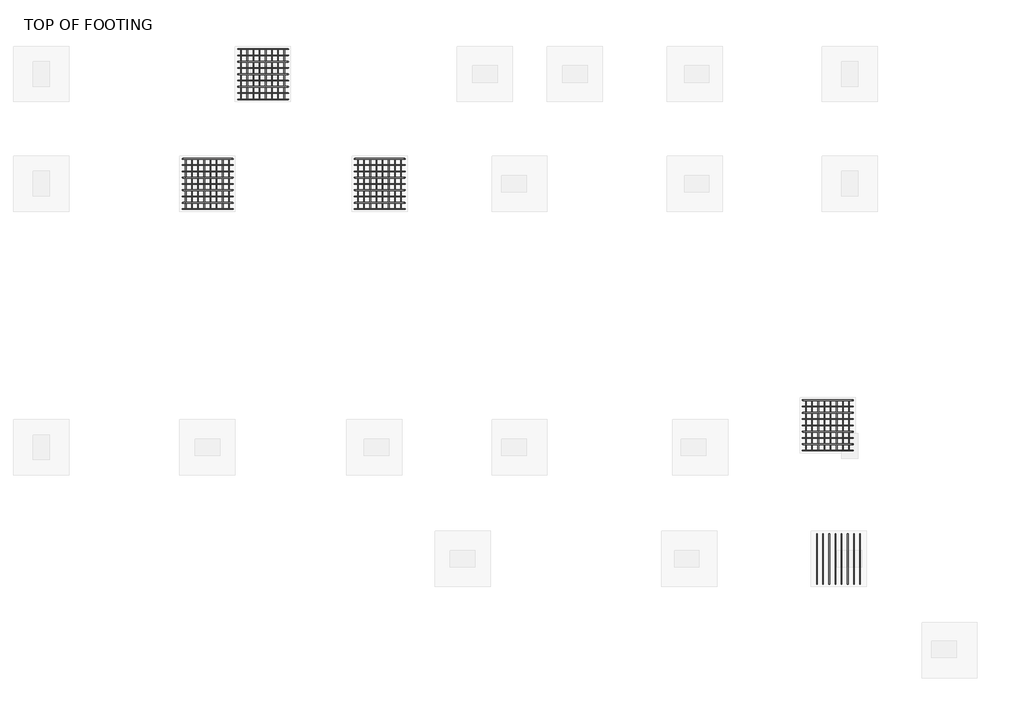
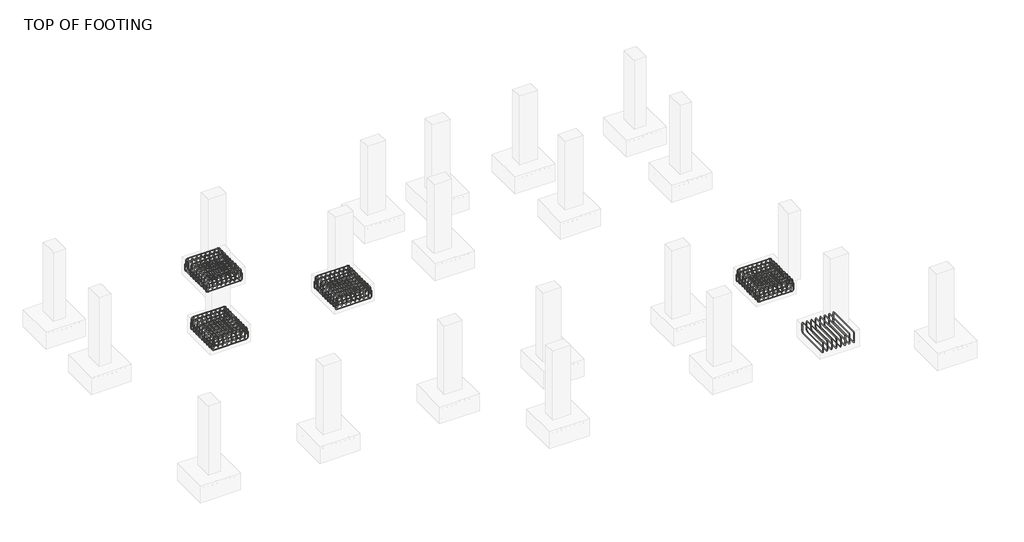
# One storey, part 16 of 20: 18 reinforcing bars.
"""IFC4 building model written with IfcOpenShell, lengths in millimetres."""

from ifc_helpers import new_model, si_unit, point, frame, origin, place, context, project, spatial, polyline, circle_curve, trimmed, segment, composite_curve, source, transform, mapped, element, save
from ifc_brep_helpers import swept_disk

model = new_model("IFC4")

# Units and contexts
model_context = context("Model", 3, world=origin())
ifc_project = project(units=[si_unit("LENGTHUNIT", "METRE", prefix="MILLI")], contexts=[model_context])

# Site, building, storey
site = spatial("IfcSite", under=ifc_project)
building = spatial("IfcBuilding", under=site)
storey = spatial("IfcBuildingStorey", under=building, Name="TOP OF FOOTING", Elevation=-1828.8)

# Reinforcing bars
placement = place(None, origin())
reinforcing_bar_shape = source(origin(), model_context, "Body", "SolidModel", [
    swept_disk(composite_curve([segment(polyline([(4736.1748054, 12461.0575451, -2006.6587682), (4736.1748054, 12461.0575451, -2153.9587682)]), True, "CONTINUOUS"), segment(trimmed(circle_curve(frame((4689.8248054, 12461.0575451, -2153.9587682), z_axis=(0.0, 1.0, 0.0), x_axis=(46.350000000000364, 0.0, 0.0)), 46.35), [point((4736.1748054, 12461.0575451, -2153.9587682))], [point((4689.8248054, 12461.0575451, -2200.3087682))], True, "CARTESIAN"), True, "CONTINUOUS"), segment(polyline([(4689.8248054, 12461.0575451, -2200.3087682), (3875.2248054, 12461.0575451, -2200.3087682)]), True, "CONTINUOUS"), segment(trimmed(circle_curve(frame((3875.2248054, 12461.0575451, -2153.9587682), z_axis=(0.0, 1.0, 0.0), x_axis=(0.0, 0.0, -46.34999999999991)), 46.35), [point((3875.2248054, 12461.0575451, -2200.3087682))], [point((3828.8748054, 12461.0575451, -2153.9587682))], True, "CARTESIAN"), True, "CONTINUOUS"), segment(polyline([(3828.8748054, 12461.0575451, -2153.9587682), (3828.8748054, 12461.0575451, -2006.6587682)]), True, "CONTINUOUS")], self_intersect=False), 6.35),
])
element("IfcReinforcingBar", 1, at=placement, inside=storey, context=model_context, shape_type="MappedRepresentation", body=[
    mapped(reinforcing_bar_shape, transform((0.0, 0.0, 0.0), x_axis=(1.0, 0.0, 0.0), y_axis=(0.0, 1.0, 0.0), z_axis=(0.0, 0.0, 1.0))),
    mapped(reinforcing_bar_shape, transform((0.0, -113.4125, 0.0), x_axis=(1.0, 0.0, 0.0), y_axis=(0.0, 1.0, 0.0), z_axis=(0.0, 0.0, 1.0))),
    mapped(reinforcing_bar_shape, transform((0.0, -226.825, 0.0), x_axis=(1.0, 0.0, 0.0), y_axis=(0.0, 1.0, 0.0), z_axis=(0.0, 0.0, 1.0))),
    mapped(reinforcing_bar_shape, transform((0.0, -340.2375, 0.0), x_axis=(1.0, 0.0, 0.0), y_axis=(0.0, 1.0, 0.0), z_axis=(0.0, 0.0, 1.0))),
    mapped(reinforcing_bar_shape, transform((0.0, -453.65, 0.0), x_axis=(1.0, 0.0, 0.0), y_axis=(0.0, 1.0, 0.0), z_axis=(0.0, 0.0, 1.0))),
    mapped(reinforcing_bar_shape, transform((0.0, -567.0625, 0.0), x_axis=(1.0, 0.0, 0.0), y_axis=(0.0, 1.0, 0.0), z_axis=(0.0, 0.0, 1.0))),
    mapped(reinforcing_bar_shape, transform((0.0, -680.475, 0.0), x_axis=(1.0, 0.0, 0.0), y_axis=(0.0, 1.0, 0.0), z_axis=(0.0, 0.0, 1.0))),
    mapped(reinforcing_bar_shape, transform((0.0, -793.8875, 0.0), x_axis=(1.0, 0.0, 0.0), y_axis=(0.0, 1.0, 0.0), z_axis=(0.0, 0.0, 1.0))),
    mapped(reinforcing_bar_shape, transform((0.0, -907.3, 0.0), x_axis=(1.0, 0.0, 0.0), y_axis=(0.0, 1.0, 0.0), z_axis=(0.0, 0.0, 1.0))),
])
reinforcing_bar_2_shape = source(origin(), model_context, "Body", "SolidModel", [
    swept_disk(composite_curve([segment(polyline([(3848.3489167, 12461.0575451, -2068.8), (3848.3489167, 12461.0575451, -1921.5)]), True, "CONTINUOUS"), segment(trimmed(circle_curve(frame((3894.6989167, 12461.0575451, -1921.5), z_axis=(0.0, 1.0, 0.0), x_axis=(-46.350000000000364, 0.0, 0.0)), 46.35), [point((3848.3489167, 12461.0575451, -1921.5))], [point((3894.6989167, 12461.0575451, -1875.15))], True, "CARTESIAN"), True, "CONTINUOUS"), segment(polyline([(3894.6989167, 12461.0575451, -1875.15), (4664.1623164, 12461.0575451, -1875.15)]), True, "CONTINUOUS"), segment(trimmed(circle_curve(frame((4664.1623164, 12461.0575451, -1921.5), z_axis=(0.0, 1.0, 0.0), x_axis=(0.0, 0.0, 46.34999999999991)), 46.35), [point((4664.1623164, 12461.0575451, -1875.15))], [point((4710.5123164, 12461.0575451, -1921.5))], True, "CARTESIAN"), True, "CONTINUOUS"), segment(polyline([(4710.5123164, 12461.0575451, -1921.5), (4710.5123164, 12461.0575451, -2068.8)]), True, "CONTINUOUS")], self_intersect=False), 6.35),
])
element("IfcReinforcingBar", 2, at=placement, inside=storey, context=model_context, shape_type="MappedRepresentation", body=[
    mapped(reinforcing_bar_2_shape, transform((0.0, 0.0, 0.0), x_axis=(1.0, 0.0, 0.0), y_axis=(0.0, 1.0, 0.0), z_axis=(0.0, 0.0, 1.0))),
    mapped(reinforcing_bar_2_shape, transform((0.0, -113.4125, 0.0), x_axis=(1.0, 0.0, 0.0), y_axis=(0.0, 1.0, 0.0), z_axis=(0.0, 0.0, 1.0))),
    mapped(reinforcing_bar_2_shape, transform((0.0, -226.825, 0.0), x_axis=(1.0, 0.0, 0.0), y_axis=(0.0, 1.0, 0.0), z_axis=(0.0, 0.0, 1.0))),
    mapped(reinforcing_bar_2_shape, transform((0.0, -340.2375, 0.0), x_axis=(1.0, 0.0, 0.0), y_axis=(0.0, 1.0, 0.0), z_axis=(0.0, 0.0, 1.0))),
    mapped(reinforcing_bar_2_shape, transform((0.0, -453.65, 0.0), x_axis=(1.0, 0.0, 0.0), y_axis=(0.0, 1.0, 0.0), z_axis=(0.0, 0.0, 1.0))),
    mapped(reinforcing_bar_2_shape, transform((0.0, -567.0625, 0.0), x_axis=(1.0, 0.0, 0.0), y_axis=(0.0, 1.0, 0.0), z_axis=(0.0, 0.0, 1.0))),
    mapped(reinforcing_bar_2_shape, transform((0.0, -680.475, 0.0), x_axis=(1.0, 0.0, 0.0), y_axis=(0.0, 1.0, 0.0), z_axis=(0.0, 0.0, 1.0))),
    mapped(reinforcing_bar_2_shape, transform((0.0, -793.8875, 0.0), x_axis=(1.0, 0.0, 0.0), y_axis=(0.0, 1.0, 0.0), z_axis=(0.0, 0.0, 1.0))),
    mapped(reinforcing_bar_2_shape, transform((0.0, -907.3, 0.0), x_axis=(1.0, 0.0, 0.0), y_axis=(0.0, 1.0, 0.0), z_axis=(0.0, 0.0, 1.0))),
])
reinforcing_bar_3_shape = source(origin(), model_context, "Body", "SolidModel", [
    swept_disk(composite_curve([segment(polyline([(4664.677844, 12461.0575451, -2086.1951968), (4664.677844, 12461.0575451, -1938.8951968)]), True, "CONTINUOUS"), segment(trimmed(circle_curve(frame((4664.677844, 12414.7075451, -1938.8951968), z_axis=(1.0, 0.0, 0.0), x_axis=(0.0, 46.350000000000364, 0.0)), 46.35), [point((4664.677844, 12461.0575451, -1938.8951968))], [point((4664.677844, 12414.7075451, -1892.5451968))], True, "CARTESIAN"), True, "CONTINUOUS"), segment(polyline([(4664.677844, 12414.7075451, -1892.5451968), (4664.677844, 11600.1075451, -1892.5451968)]), True, "CONTINUOUS"), segment(trimmed(circle_curve(frame((4664.677844, 11600.1075451, -1938.8951968), z_axis=(1.0, 0.0, 0.0), x_axis=(0.0, 0.0, 46.34999999999991)), 46.35), [point((4664.677844, 11600.1075451, -1892.5451968))], [point((4664.677844, 11553.7575451, -1938.8951968))], True, "CARTESIAN"), True, "CONTINUOUS"), segment(polyline([(4664.677844, 11553.7575451, -1938.8951968), (4664.677844, 11553.7575451, -2086.1951968)]), True, "CONTINUOUS")], self_intersect=False), 6.35),
])
element("IfcReinforcingBar", 3, at=placement, inside=storey, context=model_context, shape_type="MappedRepresentation", body=[
    mapped(reinforcing_bar_3_shape, transform((0.0, 0.0, 0.0), x_axis=(1.0, 0.0, 0.0), y_axis=(0.0, 1.0, 0.0), z_axis=(0.0, 0.0, 1.0))),
    mapped(reinforcing_bar_3_shape, transform((-111.2862402, 0.0, 0.0), x_axis=(1.0, 0.0, 0.0), y_axis=(0.0, 1.0, 0.0), z_axis=(0.0, 0.0, 1.0))),
    mapped(reinforcing_bar_3_shape, transform((-222.5724804, 0.0, 0.0), x_axis=(1.0, 0.0, 0.0), y_axis=(0.0, 1.0, 0.0), z_axis=(0.0, 0.0, 1.0))),
    mapped(reinforcing_bar_3_shape, transform((-333.8587205, 0.0, 0.0), x_axis=(1.0, 0.0, 0.0), y_axis=(0.0, 1.0, 0.0), z_axis=(0.0, 0.0, 1.0))),
    mapped(reinforcing_bar_3_shape, transform((-445.1449607, 0.0, 0.0), x_axis=(1.0, 0.0, 0.0), y_axis=(0.0, 1.0, 0.0), z_axis=(0.0, 0.0, 1.0))),
    mapped(reinforcing_bar_3_shape, transform((-556.4312009, 0.0, 0.0), x_axis=(1.0, 0.0, 0.0), y_axis=(0.0, 1.0, 0.0), z_axis=(0.0, 0.0, 1.0))),
    mapped(reinforcing_bar_3_shape, transform((-667.7174411, 0.0, 0.0), x_axis=(1.0, 0.0, 0.0), y_axis=(0.0, 1.0, 0.0), z_axis=(0.0, 0.0, 1.0))),
    mapped(reinforcing_bar_3_shape, transform((-779.0036813, 0.0, 0.0), x_axis=(1.0, 0.0, 0.0), y_axis=(0.0, 1.0, 0.0), z_axis=(0.0, 0.0, 1.0))),
])
reinforcing_bar_4_shape = source(origin(), model_context, "Body", "SolidModel", [
    swept_disk(composite_curve([segment(polyline([(3885.6741627, 12461.0575451, -1979.1645013), (3885.6741627, 12461.0575451, -2126.4645013)]), True, "CONTINUOUS"), segment(trimmed(circle_curve(frame((3885.6741627, 12414.7075451, -2126.4645013), z_axis=(-1.0, 0.0, 0.0), x_axis=(0.0, 46.350000000000364, 0.0)), 46.35), [point((3885.6741627, 12461.0575451, -2126.4645013))], [point((3885.6741627, 12414.7075451, -2172.8145013))], True, "CARTESIAN"), True, "CONTINUOUS"), segment(polyline([(3885.6741627, 12414.7075451, -2172.8145013), (3885.6741627, 11600.1075451, -2172.8145013)]), True, "CONTINUOUS"), segment(trimmed(circle_curve(frame((3885.6741627, 11600.1075451, -2126.4645013), z_axis=(-1.0, 0.0, 0.0), x_axis=(0.0, 0.0, -46.34999999999991)), 46.35), [point((3885.6741627, 11600.1075451, -2172.8145013))], [point((3885.6741627, 11553.7575451, -2126.4645013))], True, "CARTESIAN"), True, "CONTINUOUS"), segment(polyline([(3885.6741627, 11553.7575451, -2126.4645013), (3885.6741627, 11553.7575451, -1979.1645013)]), True, "CONTINUOUS")], self_intersect=False), 6.35),
])
element("IfcReinforcingBar", 4, at=placement, inside=storey, context=model_context, shape_type="MappedRepresentation", body=[
    mapped(reinforcing_bar_4_shape, transform((0.0, 0.0, 0.0), x_axis=(1.0, 0.0, 0.0), y_axis=(0.0, 1.0, 0.0), z_axis=(0.0, 0.0, 1.0))),
    mapped(reinforcing_bar_4_shape, transform((111.2862402, 0.0, 0.0), x_axis=(1.0, 0.0, 0.0), y_axis=(0.0, 1.0, 0.0), z_axis=(0.0, 0.0, 1.0))),
    mapped(reinforcing_bar_4_shape, transform((222.5724804, 0.0, 0.0), x_axis=(1.0, 0.0, 0.0), y_axis=(0.0, 1.0, 0.0), z_axis=(0.0, 0.0, 1.0))),
    mapped(reinforcing_bar_4_shape, transform((333.8587205, 0.0, 0.0), x_axis=(1.0, 0.0, 0.0), y_axis=(0.0, 1.0, 0.0), z_axis=(0.0, 0.0, 1.0))),
    mapped(reinforcing_bar_4_shape, transform((445.1449607, 0.0, 0.0), x_axis=(1.0, 0.0, 0.0), y_axis=(0.0, 1.0, 0.0), z_axis=(0.0, 0.0, 1.0))),
    mapped(reinforcing_bar_4_shape, transform((556.4312009, 0.0, 0.0), x_axis=(1.0, 0.0, 0.0), y_axis=(0.0, 1.0, 0.0), z_axis=(0.0, 0.0, 1.0))),
    mapped(reinforcing_bar_4_shape, transform((667.7174411, 0.0, 0.0), x_axis=(1.0, 0.0, 0.0), y_axis=(0.0, 1.0, 0.0), z_axis=(0.0, 0.0, 1.0))),
    mapped(reinforcing_bar_4_shape, transform((779.0036813, 0.0, 0.0), x_axis=(1.0, 0.0, 0.0), y_axis=(0.0, 1.0, 0.0), z_axis=(0.0, 0.0, 1.0))),
])
reinforcing_bar_5_shape = source(origin(), model_context, "Body", "SolidModel", [
    swept_disk(composite_curve([segment(polyline([(2628.3796816, 14441.1679708, -2006.6587682), (2628.3796816, 14441.1679708, -2153.9587682)]), True, "CONTINUOUS"), segment(trimmed(circle_curve(frame((2582.0296816, 14441.1679708, -2153.9587682), z_axis=(0.0, 1.0, 0.0), x_axis=(46.34999999999991, 0.0, 0.0)), 46.35), [point((2628.3796816, 14441.1679708, -2153.9587682))], [point((2582.0296816, 14441.1679708, -2200.3087682))], True, "CARTESIAN"), True, "CONTINUOUS"), segment(polyline([(2582.0296816, 14441.1679708, -2200.3087682), (1767.4296816, 14441.1679708, -2200.3087682)]), True, "CONTINUOUS"), segment(trimmed(circle_curve(frame((1767.4296816, 14441.1679708, -2153.9587682), z_axis=(0.0, 1.0, 0.0), x_axis=(0.0, 0.0, -46.34999999999991)), 46.35), [point((1767.4296816, 14441.1679708, -2200.3087682))], [point((1721.0796816, 14441.1679708, -2153.9587682))], True, "CARTESIAN"), True, "CONTINUOUS"), segment(polyline([(1721.0796816, 14441.1679708, -2153.9587682), (1721.0796816, 14441.1679708, -2006.6587682)]), True, "CONTINUOUS")], self_intersect=False), 6.35),
])
element("IfcReinforcingBar", 5, at=placement, inside=storey, context=model_context, shape_type="MappedRepresentation", body=[
    mapped(reinforcing_bar_5_shape, transform((0.0, 0.0, 0.0), x_axis=(1.0, 0.0, 0.0), y_axis=(0.0, 1.0, 0.0), z_axis=(0.0, 0.0, 1.0))),
    mapped(reinforcing_bar_5_shape, transform((0.0, -113.4125, 0.0), x_axis=(1.0, 0.0, 0.0), y_axis=(0.0, 1.0, 0.0), z_axis=(0.0, 0.0, 1.0))),
    mapped(reinforcing_bar_5_shape, transform((0.0, -226.825, 0.0), x_axis=(1.0, 0.0, 0.0), y_axis=(0.0, 1.0, 0.0), z_axis=(0.0, 0.0, 1.0))),
    mapped(reinforcing_bar_5_shape, transform((0.0, -340.2375, 0.0), x_axis=(1.0, 0.0, 0.0), y_axis=(0.0, 1.0, 0.0), z_axis=(0.0, 0.0, 1.0))),
    mapped(reinforcing_bar_5_shape, transform((0.0, -453.65, 0.0), x_axis=(1.0, 0.0, 0.0), y_axis=(0.0, 1.0, 0.0), z_axis=(0.0, 0.0, 1.0))),
    mapped(reinforcing_bar_5_shape, transform((0.0, -567.0625, 0.0), x_axis=(1.0, 0.0, 0.0), y_axis=(0.0, 1.0, 0.0), z_axis=(0.0, 0.0, 1.0))),
    mapped(reinforcing_bar_5_shape, transform((0.0, -680.475, 0.0), x_axis=(1.0, 0.0, 0.0), y_axis=(0.0, 1.0, 0.0), z_axis=(0.0, 0.0, 1.0))),
    mapped(reinforcing_bar_5_shape, transform((0.0, -793.8875, 0.0), x_axis=(1.0, 0.0, 0.0), y_axis=(0.0, 1.0, 0.0), z_axis=(0.0, 0.0, 1.0))),
    mapped(reinforcing_bar_5_shape, transform((0.0, -907.3, 0.0), x_axis=(1.0, 0.0, 0.0), y_axis=(0.0, 1.0, 0.0), z_axis=(0.0, 0.0, 1.0))),
])
reinforcing_bar_6_shape = source(origin(), model_context, "Body", "SolidModel", [
    swept_disk(composite_curve([segment(polyline([(1740.553793, 14441.1679708, -2068.8), (1740.553793, 14441.1679708, -1921.5)]), True, "CONTINUOUS"), segment(trimmed(circle_curve(frame((1786.903793, 14441.1679708, -1921.5), z_axis=(0.0, 1.0, 0.0), x_axis=(-46.34999999999991, 0.0, 0.0)), 46.35), [point((1740.553793, 14441.1679708, -1921.5))], [point((1786.903793, 14441.1679708, -1875.15))], True, "CARTESIAN"), True, "CONTINUOUS"), segment(polyline([(1786.903793, 14441.1679708, -1875.15), (2556.3671926, 14441.1679708, -1875.15)]), True, "CONTINUOUS"), segment(trimmed(circle_curve(frame((2556.3671926, 14441.1679708, -1921.5), z_axis=(0.0, 1.0, 0.0), x_axis=(0.0, 0.0, 46.34999999999991)), 46.35), [point((2556.3671926, 14441.1679708, -1875.15))], [point((2602.7171926, 14441.1679708, -1921.5))], True, "CARTESIAN"), True, "CONTINUOUS"), segment(polyline([(2602.7171926, 14441.1679708, -1921.5), (2602.7171926, 14441.1679708, -2068.8)]), True, "CONTINUOUS")], self_intersect=False), 6.35),
])
element("IfcReinforcingBar", 6, at=placement, inside=storey, context=model_context, shape_type="MappedRepresentation", body=[
    mapped(reinforcing_bar_6_shape, transform((0.0, 0.0, 0.0), x_axis=(1.0, 0.0, 0.0), y_axis=(0.0, 1.0, 0.0), z_axis=(0.0, 0.0, 1.0))),
    mapped(reinforcing_bar_6_shape, transform((0.0, -113.4125, 0.0), x_axis=(1.0, 0.0, 0.0), y_axis=(0.0, 1.0, 0.0), z_axis=(0.0, 0.0, 1.0))),
    mapped(reinforcing_bar_6_shape, transform((0.0, -226.825, 0.0), x_axis=(1.0, 0.0, 0.0), y_axis=(0.0, 1.0, 0.0), z_axis=(0.0, 0.0, 1.0))),
    mapped(reinforcing_bar_6_shape, transform((0.0, -340.2375, 0.0), x_axis=(1.0, 0.0, 0.0), y_axis=(0.0, 1.0, 0.0), z_axis=(0.0, 0.0, 1.0))),
    mapped(reinforcing_bar_6_shape, transform((0.0, -453.65, 0.0), x_axis=(1.0, 0.0, 0.0), y_axis=(0.0, 1.0, 0.0), z_axis=(0.0, 0.0, 1.0))),
    mapped(reinforcing_bar_6_shape, transform((0.0, -567.0625, 0.0), x_axis=(1.0, 0.0, 0.0), y_axis=(0.0, 1.0, 0.0), z_axis=(0.0, 0.0, 1.0))),
    mapped(reinforcing_bar_6_shape, transform((0.0, -680.475, 0.0), x_axis=(1.0, 0.0, 0.0), y_axis=(0.0, 1.0, 0.0), z_axis=(0.0, 0.0, 1.0))),
    mapped(reinforcing_bar_6_shape, transform((0.0, -793.8875, 0.0), x_axis=(1.0, 0.0, 0.0), y_axis=(0.0, 1.0, 0.0), z_axis=(0.0, 0.0, 1.0))),
    mapped(reinforcing_bar_6_shape, transform((0.0, -907.3, 0.0), x_axis=(1.0, 0.0, 0.0), y_axis=(0.0, 1.0, 0.0), z_axis=(0.0, 0.0, 1.0))),
])
reinforcing_bar_7_shape = source(origin(), model_context, "Body", "SolidModel", [
    swept_disk(composite_curve([segment(polyline([(2556.8827202, 14441.1679708, -2086.1951968), (2556.8827202, 14441.1679708, -1938.8951968)]), True, "CONTINUOUS"), segment(trimmed(circle_curve(frame((2556.8827202, 14394.8179708, -1938.8951968), z_axis=(1.0, 0.0, 0.0), x_axis=(0.0, 46.349999999998545, 0.0)), 46.35), [point((2556.8827202, 14441.1679708, -1938.8951968))], [point((2556.8827202, 14394.8179708, -1892.5451968))], True, "CARTESIAN"), True, "CONTINUOUS"), segment(polyline([(2556.8827202, 14394.8179708, -1892.5451968), (2556.8827202, 13580.2179708, -1892.5451968)]), True, "CONTINUOUS"), segment(trimmed(circle_curve(frame((2556.8827202, 13580.2179708, -1938.8951968), z_axis=(1.0, 0.0, 0.0), x_axis=(0.0, 0.0, 46.34999999999991)), 46.35), [point((2556.8827202, 13580.2179708, -1892.5451968))], [point((2556.8827202, 13533.8679708, -1938.8951968))], True, "CARTESIAN"), True, "CONTINUOUS"), segment(polyline([(2556.8827202, 13533.8679708, -1938.8951968), (2556.8827202, 13533.8679708, -2086.1951968)]), True, "CONTINUOUS")], self_intersect=False), 6.35),
])
element("IfcReinforcingBar", 7, at=placement, inside=storey, context=model_context, shape_type="MappedRepresentation", body=[
    mapped(reinforcing_bar_7_shape, transform((0.0, 0.0, 0.0), x_axis=(1.0, 0.0, 0.0), y_axis=(0.0, 1.0, 0.0), z_axis=(0.0, 0.0, 1.0))),
    mapped(reinforcing_bar_7_shape, transform((-111.2862402, 0.0, 0.0), x_axis=(1.0, 0.0, 0.0), y_axis=(0.0, 1.0, 0.0), z_axis=(0.0, 0.0, 1.0))),
    mapped(reinforcing_bar_7_shape, transform((-222.5724804, 0.0, 0.0), x_axis=(1.0, 0.0, 0.0), y_axis=(0.0, 1.0, 0.0), z_axis=(0.0, 0.0, 1.0))),
    mapped(reinforcing_bar_7_shape, transform((-333.8587205, 0.0, 0.0), x_axis=(1.0, 0.0, 0.0), y_axis=(0.0, 1.0, 0.0), z_axis=(0.0, 0.0, 1.0))),
    mapped(reinforcing_bar_7_shape, transform((-445.1449607, 0.0, 0.0), x_axis=(1.0, 0.0, 0.0), y_axis=(0.0, 1.0, 0.0), z_axis=(0.0, 0.0, 1.0))),
    mapped(reinforcing_bar_7_shape, transform((-556.4312009, 0.0, 0.0), x_axis=(1.0, 0.0, 0.0), y_axis=(0.0, 1.0, 0.0), z_axis=(0.0, 0.0, 1.0))),
    mapped(reinforcing_bar_7_shape, transform((-667.7174411, 0.0, 0.0), x_axis=(1.0, 0.0, 0.0), y_axis=(0.0, 1.0, 0.0), z_axis=(0.0, 0.0, 1.0))),
    mapped(reinforcing_bar_7_shape, transform((-779.0036813, 0.0, 0.0), x_axis=(1.0, 0.0, 0.0), y_axis=(0.0, 1.0, 0.0), z_axis=(0.0, 0.0, 1.0))),
])
reinforcing_bar_8_shape = source(origin(), model_context, "Body", "SolidModel", [
    swept_disk(composite_curve([segment(polyline([(1777.879039, 14441.1679708, -1979.1645013), (1777.879039, 14441.1679708, -2126.4645013)]), True, "CONTINUOUS"), segment(trimmed(circle_curve(frame((1777.879039, 14394.8179708, -2126.4645013), z_axis=(-1.0, 0.0, 0.0), x_axis=(0.0, 46.349999999998545, 0.0)), 46.35), [point((1777.879039, 14441.1679708, -2126.4645013))], [point((1777.879039, 14394.8179708, -2172.8145013))], True, "CARTESIAN"), True, "CONTINUOUS"), segment(polyline([(1777.879039, 14394.8179708, -2172.8145013), (1777.879039, 13580.2179708, -2172.8145013)]), True, "CONTINUOUS"), segment(trimmed(circle_curve(frame((1777.879039, 13580.2179708, -2126.4645013), z_axis=(-1.0, 0.0, 0.0), x_axis=(0.0, 0.0, -46.34999999999991)), 46.35), [point((1777.879039, 13580.2179708, -2172.8145013))], [point((1777.879039, 13533.8679708, -2126.4645013))], True, "CARTESIAN"), True, "CONTINUOUS"), segment(polyline([(1777.879039, 13533.8679708, -2126.4645013), (1777.879039, 13533.8679708, -1979.1645013)]), True, "CONTINUOUS")], self_intersect=False), 6.35),
])
element("IfcReinforcingBar", 8, at=placement, inside=storey, context=model_context, shape_type="MappedRepresentation", body=[
    mapped(reinforcing_bar_8_shape, transform((0.0, 0.0, 0.0), x_axis=(1.0, 0.0, 0.0), y_axis=(0.0, 1.0, 0.0), z_axis=(0.0, 0.0, 1.0))),
    mapped(reinforcing_bar_8_shape, transform((111.2862402, 0.0, 0.0), x_axis=(1.0, 0.0, 0.0), y_axis=(0.0, 1.0, 0.0), z_axis=(0.0, 0.0, 1.0))),
    mapped(reinforcing_bar_8_shape, transform((222.5724804, 0.0, 0.0), x_axis=(1.0, 0.0, 0.0), y_axis=(0.0, 1.0, 0.0), z_axis=(0.0, 0.0, 1.0))),
    mapped(reinforcing_bar_8_shape, transform((333.8587205, 0.0, 0.0), x_axis=(1.0, 0.0, 0.0), y_axis=(0.0, 1.0, 0.0), z_axis=(0.0, 0.0, 1.0))),
    mapped(reinforcing_bar_8_shape, transform((445.1449607, 0.0, 0.0), x_axis=(1.0, 0.0, 0.0), y_axis=(0.0, 1.0, 0.0), z_axis=(0.0, 0.0, 1.0))),
    mapped(reinforcing_bar_8_shape, transform((556.4312009, 0.0, 0.0), x_axis=(1.0, 0.0, 0.0), y_axis=(0.0, 1.0, 0.0), z_axis=(0.0, 0.0, 1.0))),
    mapped(reinforcing_bar_8_shape, transform((667.7174411, 0.0, 0.0), x_axis=(1.0, 0.0, 0.0), y_axis=(0.0, 1.0, 0.0), z_axis=(0.0, 0.0, 1.0))),
    mapped(reinforcing_bar_8_shape, transform((779.0036813, 0.0, 0.0), x_axis=(1.0, 0.0, 0.0), y_axis=(0.0, 1.0, 0.0), z_axis=(0.0, 0.0, 1.0))),
])
reinforcing_bar_9_shape = source(origin(), model_context, "Body", "SolidModel", [
    swept_disk(composite_curve([segment(polyline([(1628.3796816, 12461.0575451, -2006.6587682), (1628.3796816, 12461.0575451, -2153.9587682)]), True, "CONTINUOUS"), segment(trimmed(circle_curve(frame((1582.0296816, 12461.0575451, -2153.9587682), z_axis=(0.0, 1.0, 0.0), x_axis=(46.34999999999991, 0.0, 0.0)), 46.35), [point((1628.3796816, 12461.0575451, -2153.9587682))], [point((1582.0296816, 12461.0575451, -2200.3087682))], True, "CARTESIAN"), True, "CONTINUOUS"), segment(polyline([(1582.0296816, 12461.0575451, -2200.3087682), (767.4296816, 12461.0575451, -2200.3087682)]), True, "CONTINUOUS"), segment(trimmed(circle_curve(frame((767.4296816, 12461.0575451, -2153.9587682), z_axis=(0.0, 1.0, 0.0), x_axis=(0.0, 0.0, -46.34999999999991)), 46.35), [point((767.4296816, 12461.0575451, -2200.3087682))], [point((721.0796816, 12461.0575451, -2153.9587682))], True, "CARTESIAN"), True, "CONTINUOUS"), segment(polyline([(721.0796816, 12461.0575451, -2153.9587682), (721.0796816, 12461.0575451, -2006.6587682)]), True, "CONTINUOUS")], self_intersect=False), 6.35),
])
element("IfcReinforcingBar", 9, at=placement, inside=storey, context=model_context, shape_type="MappedRepresentation", body=[
    mapped(reinforcing_bar_9_shape, transform((0.0, 0.0, 0.0), x_axis=(1.0, 0.0, 0.0), y_axis=(0.0, 1.0, 0.0), z_axis=(0.0, 0.0, 1.0))),
    mapped(reinforcing_bar_9_shape, transform((0.0, -113.4125, 0.0), x_axis=(1.0, 0.0, 0.0), y_axis=(0.0, 1.0, 0.0), z_axis=(0.0, 0.0, 1.0))),
    mapped(reinforcing_bar_9_shape, transform((0.0, -226.825, 0.0), x_axis=(1.0, 0.0, 0.0), y_axis=(0.0, 1.0, 0.0), z_axis=(0.0, 0.0, 1.0))),
    mapped(reinforcing_bar_9_shape, transform((0.0, -340.2375, 0.0), x_axis=(1.0, 0.0, 0.0), y_axis=(0.0, 1.0, 0.0), z_axis=(0.0, 0.0, 1.0))),
    mapped(reinforcing_bar_9_shape, transform((0.0, -453.65, 0.0), x_axis=(1.0, 0.0, 0.0), y_axis=(0.0, 1.0, 0.0), z_axis=(0.0, 0.0, 1.0))),
    mapped(reinforcing_bar_9_shape, transform((0.0, -567.0625, 0.0), x_axis=(1.0, 0.0, 0.0), y_axis=(0.0, 1.0, 0.0), z_axis=(0.0, 0.0, 1.0))),
    mapped(reinforcing_bar_9_shape, transform((0.0, -680.475, 0.0), x_axis=(1.0, 0.0, 0.0), y_axis=(0.0, 1.0, 0.0), z_axis=(0.0, 0.0, 1.0))),
    mapped(reinforcing_bar_9_shape, transform((0.0, -793.8875, 0.0), x_axis=(1.0, 0.0, 0.0), y_axis=(0.0, 1.0, 0.0), z_axis=(0.0, 0.0, 1.0))),
    mapped(reinforcing_bar_9_shape, transform((0.0, -907.3, 0.0), x_axis=(1.0, 0.0, 0.0), y_axis=(0.0, 1.0, 0.0), z_axis=(0.0, 0.0, 1.0))),
])
reinforcing_bar_10_shape = source(origin(), model_context, "Body", "SolidModel", [
    swept_disk(composite_curve([segment(polyline([(740.553793, 12461.0575451, -2068.8), (740.553793, 12461.0575451, -1921.5)]), True, "CONTINUOUS"), segment(trimmed(circle_curve(frame((786.903793, 12461.0575451, -1921.5), z_axis=(0.0, 1.0, 0.0), x_axis=(-46.34999999999991, 0.0, 0.0)), 46.35), [point((740.553793, 12461.0575451, -1921.5))], [point((786.903793, 12461.0575451, -1875.15))], True, "CARTESIAN"), True, "CONTINUOUS"), segment(polyline([(786.903793, 12461.0575451, -1875.15), (1556.3671926, 12461.0575451, -1875.15)]), True, "CONTINUOUS"), segment(trimmed(circle_curve(frame((1556.3671926, 12461.0575451, -1921.5), z_axis=(0.0, 1.0, 0.0), x_axis=(0.0, 0.0, 46.34999999999991)), 46.35), [point((1556.3671926, 12461.0575451, -1875.15))], [point((1602.7171926, 12461.0575451, -1921.5))], True, "CARTESIAN"), True, "CONTINUOUS"), segment(polyline([(1602.7171926, 12461.0575451, -1921.5), (1602.7171926, 12461.0575451, -2068.8)]), True, "CONTINUOUS")], self_intersect=False), 6.35),
])
element("IfcReinforcingBar", 10, at=placement, inside=storey, context=model_context, shape_type="MappedRepresentation", body=[
    mapped(reinforcing_bar_10_shape, transform((0.0, 0.0, 0.0), x_axis=(1.0, 0.0, 0.0), y_axis=(0.0, 1.0, 0.0), z_axis=(0.0, 0.0, 1.0))),
    mapped(reinforcing_bar_10_shape, transform((0.0, -113.4125, 0.0), x_axis=(1.0, 0.0, 0.0), y_axis=(0.0, 1.0, 0.0), z_axis=(0.0, 0.0, 1.0))),
    mapped(reinforcing_bar_10_shape, transform((0.0, -226.825, 0.0), x_axis=(1.0, 0.0, 0.0), y_axis=(0.0, 1.0, 0.0), z_axis=(0.0, 0.0, 1.0))),
    mapped(reinforcing_bar_10_shape, transform((0.0, -340.2375, 0.0), x_axis=(1.0, 0.0, 0.0), y_axis=(0.0, 1.0, 0.0), z_axis=(0.0, 0.0, 1.0))),
    mapped(reinforcing_bar_10_shape, transform((0.0, -453.65, 0.0), x_axis=(1.0, 0.0, 0.0), y_axis=(0.0, 1.0, 0.0), z_axis=(0.0, 0.0, 1.0))),
    mapped(reinforcing_bar_10_shape, transform((0.0, -567.0625, 0.0), x_axis=(1.0, 0.0, 0.0), y_axis=(0.0, 1.0, 0.0), z_axis=(0.0, 0.0, 1.0))),
    mapped(reinforcing_bar_10_shape, transform((0.0, -680.475, 0.0), x_axis=(1.0, 0.0, 0.0), y_axis=(0.0, 1.0, 0.0), z_axis=(0.0, 0.0, 1.0))),
    mapped(reinforcing_bar_10_shape, transform((0.0, -793.8875, 0.0), x_axis=(1.0, 0.0, 0.0), y_axis=(0.0, 1.0, 0.0), z_axis=(0.0, 0.0, 1.0))),
    mapped(reinforcing_bar_10_shape, transform((0.0, -907.3, 0.0), x_axis=(1.0, 0.0, 0.0), y_axis=(0.0, 1.0, 0.0), z_axis=(0.0, 0.0, 1.0))),
])
reinforcing_bar_11_shape = source(origin(), model_context, "Body", "SolidModel", [
    swept_disk(composite_curve([segment(polyline([(1556.8827202, 12461.0575451, -2086.1951968), (1556.8827202, 12461.0575451, -1938.8951968)]), True, "CONTINUOUS"), segment(trimmed(circle_curve(frame((1556.8827202, 12414.7075451, -1938.8951968), z_axis=(1.0, 0.0, 0.0), x_axis=(0.0, 46.350000000000364, 0.0)), 46.35), [point((1556.8827202, 12461.0575451, -1938.8951968))], [point((1556.8827202, 12414.7075451, -1892.5451968))], True, "CARTESIAN"), True, "CONTINUOUS"), segment(polyline([(1556.8827202, 12414.7075451, -1892.5451968), (1556.8827202, 11600.1075451, -1892.5451968)]), True, "CONTINUOUS"), segment(trimmed(circle_curve(frame((1556.8827202, 11600.1075451, -1938.8951968), z_axis=(1.0, 0.0, 0.0), x_axis=(0.0, 0.0, 46.34999999999991)), 46.35), [point((1556.8827202, 11600.1075451, -1892.5451968))], [point((1556.8827202, 11553.7575451, -1938.8951968))], True, "CARTESIAN"), True, "CONTINUOUS"), segment(polyline([(1556.8827202, 11553.7575451, -1938.8951968), (1556.8827202, 11553.7575451, -2086.1951968)]), True, "CONTINUOUS")], self_intersect=False), 6.35),
])
element("IfcReinforcingBar", 11, at=placement, inside=storey, context=model_context, shape_type="MappedRepresentation", body=[
    mapped(reinforcing_bar_11_shape, transform((0.0, 0.0, 0.0), x_axis=(1.0, 0.0, 0.0), y_axis=(0.0, 1.0, 0.0), z_axis=(0.0, 0.0, 1.0))),
    mapped(reinforcing_bar_11_shape, transform((-111.2862402, 0.0, 0.0), x_axis=(1.0, 0.0, 0.0), y_axis=(0.0, 1.0, 0.0), z_axis=(0.0, 0.0, 1.0))),
    mapped(reinforcing_bar_11_shape, transform((-222.5724804, 0.0, 0.0), x_axis=(1.0, 0.0, 0.0), y_axis=(0.0, 1.0, 0.0), z_axis=(0.0, 0.0, 1.0))),
    mapped(reinforcing_bar_11_shape, transform((-333.8587205, 0.0, 0.0), x_axis=(1.0, 0.0, 0.0), y_axis=(0.0, 1.0, 0.0), z_axis=(0.0, 0.0, 1.0))),
    mapped(reinforcing_bar_11_shape, transform((-445.1449607, 0.0, 0.0), x_axis=(1.0, 0.0, 0.0), y_axis=(0.0, 1.0, 0.0), z_axis=(0.0, 0.0, 1.0))),
    mapped(reinforcing_bar_11_shape, transform((-556.4312009, 0.0, 0.0), x_axis=(1.0, 0.0, 0.0), y_axis=(0.0, 1.0, 0.0), z_axis=(0.0, 0.0, 1.0))),
    mapped(reinforcing_bar_11_shape, transform((-667.7174411, 0.0, 0.0), x_axis=(1.0, 0.0, 0.0), y_axis=(0.0, 1.0, 0.0), z_axis=(0.0, 0.0, 1.0))),
    mapped(reinforcing_bar_11_shape, transform((-779.0036813, 0.0, 0.0), x_axis=(1.0, 0.0, 0.0), y_axis=(0.0, 1.0, 0.0), z_axis=(0.0, 0.0, 1.0))),
])
reinforcing_bar_12_shape = source(origin(), model_context, "Body", "SolidModel", [
    swept_disk(composite_curve([segment(polyline([(777.879039, 12461.0575451, -1979.1645013), (777.879039, 12461.0575451, -2126.4645013)]), True, "CONTINUOUS"), segment(trimmed(circle_curve(frame((777.879039, 12414.7075451, -2126.4645013), z_axis=(-1.0, 0.0, 0.0), x_axis=(0.0, 46.350000000000364, 0.0)), 46.35), [point((777.879039, 12461.0575451, -2126.4645013))], [point((777.879039, 12414.7075451, -2172.8145013))], True, "CARTESIAN"), True, "CONTINUOUS"), segment(polyline([(777.879039, 12414.7075451, -2172.8145013), (777.879039, 11600.1075451, -2172.8145013)]), True, "CONTINUOUS"), segment(trimmed(circle_curve(frame((777.879039, 11600.1075451, -2126.4645013), z_axis=(-1.0, 0.0, 0.0), x_axis=(0.0, 0.0, -46.34999999999991)), 46.35), [point((777.879039, 11600.1075451, -2172.8145013))], [point((777.879039, 11553.7575451, -2126.4645013))], True, "CARTESIAN"), True, "CONTINUOUS"), segment(polyline([(777.879039, 11553.7575451, -2126.4645013), (777.879039, 11553.7575451, -1979.1645013)]), True, "CONTINUOUS")], self_intersect=False), 6.35),
])
element("IfcReinforcingBar", 12, at=placement, inside=storey, context=model_context, shape_type="MappedRepresentation", body=[
    mapped(reinforcing_bar_12_shape, transform((0.0, 0.0, 0.0), x_axis=(1.0, 0.0, 0.0), y_axis=(0.0, 1.0, 0.0), z_axis=(0.0, 0.0, 1.0))),
    mapped(reinforcing_bar_12_shape, transform((111.2862402, 0.0, 0.0), x_axis=(1.0, 0.0, 0.0), y_axis=(0.0, 1.0, 0.0), z_axis=(0.0, 0.0, 1.0))),
    mapped(reinforcing_bar_12_shape, transform((222.5724804, 0.0, 0.0), x_axis=(1.0, 0.0, 0.0), y_axis=(0.0, 1.0, 0.0), z_axis=(0.0, 0.0, 1.0))),
    mapped(reinforcing_bar_12_shape, transform((333.8587205, 0.0, 0.0), x_axis=(1.0, 0.0, 0.0), y_axis=(0.0, 1.0, 0.0), z_axis=(0.0, 0.0, 1.0))),
    mapped(reinforcing_bar_12_shape, transform((445.1449607, 0.0, 0.0), x_axis=(1.0, 0.0, 0.0), y_axis=(0.0, 1.0, 0.0), z_axis=(0.0, 0.0, 1.0))),
    mapped(reinforcing_bar_12_shape, transform((556.4312009, 0.0, 0.0), x_axis=(1.0, 0.0, 0.0), y_axis=(0.0, 1.0, 0.0), z_axis=(0.0, 0.0, 1.0))),
    mapped(reinforcing_bar_12_shape, transform((667.7174411, 0.0, 0.0), x_axis=(1.0, 0.0, 0.0), y_axis=(0.0, 1.0, 0.0), z_axis=(0.0, 0.0, 1.0))),
    mapped(reinforcing_bar_12_shape, transform((779.0036813, 0.0, 0.0), x_axis=(1.0, 0.0, 0.0), y_axis=(0.0, 1.0, 0.0), z_axis=(0.0, 0.0, 1.0))),
])
reinforcing_bar_13_shape = source(origin(), model_context, "Body", "SolidModel", [
    swept_disk(composite_curve([segment(polyline([(12822.7663908, 8103.3576276, -2006.6587682), (12822.7663908, 8103.3576276, -2153.9587682)]), True, "CONTINUOUS"), segment(trimmed(circle_curve(frame((12776.4163908, 8103.3576276, -2153.9587682), z_axis=(0.0, 1.0, 0.0), x_axis=(46.350000000000364, 0.0, 0.0)), 46.35), [point((12822.7663908, 8103.3576276, -2153.9587682))], [point((12776.4163908, 8103.3576276, -2200.3087682))], True, "CARTESIAN"), True, "CONTINUOUS"), segment(polyline([(12776.4163908, 8103.3576276, -2200.3087682), (11961.8163908, 8103.3576276, -2200.3087682)]), True, "CONTINUOUS"), segment(trimmed(circle_curve(frame((11961.8163908, 8103.3576276, -2153.9587682), z_axis=(0.0, 1.0, 0.0), x_axis=(0.0, 0.0, -46.34999999999991)), 46.35), [point((11961.8163908, 8103.3576276, -2200.3087682))], [point((11915.4663908, 8103.3576276, -2153.9587682))], True, "CARTESIAN"), True, "CONTINUOUS"), segment(polyline([(11915.4663908, 8103.3576276, -2153.9587682), (11915.4663908, 8103.3576276, -2006.6587682)]), True, "CONTINUOUS")], self_intersect=False), 6.35),
])
element("IfcReinforcingBar", 13, at=placement, inside=storey, context=model_context, shape_type="MappedRepresentation", body=[
    mapped(reinforcing_bar_13_shape, transform((0.0, 0.0, 0.0), x_axis=(1.0, 0.0, 0.0), y_axis=(0.0, 1.0, 0.0), z_axis=(0.0, 0.0, 1.0))),
    mapped(reinforcing_bar_13_shape, transform((0.0, -113.4125, 0.0), x_axis=(1.0, 0.0, 0.0), y_axis=(0.0, 1.0, 0.0), z_axis=(0.0, 0.0, 1.0))),
    mapped(reinforcing_bar_13_shape, transform((0.0, -226.825, 0.0), x_axis=(1.0, 0.0, 0.0), y_axis=(0.0, 1.0, 0.0), z_axis=(0.0, 0.0, 1.0))),
    mapped(reinforcing_bar_13_shape, transform((0.0, -340.2375, 0.0), x_axis=(1.0, 0.0, 0.0), y_axis=(0.0, 1.0, 0.0), z_axis=(0.0, 0.0, 1.0))),
    mapped(reinforcing_bar_13_shape, transform((0.0, -453.65, 0.0), x_axis=(1.0, 0.0, 0.0), y_axis=(0.0, 1.0, 0.0), z_axis=(0.0, 0.0, 1.0))),
    mapped(reinforcing_bar_13_shape, transform((0.0, -567.0625, 0.0), x_axis=(1.0, 0.0, 0.0), y_axis=(0.0, 1.0, 0.0), z_axis=(0.0, 0.0, 1.0))),
    mapped(reinforcing_bar_13_shape, transform((0.0, -680.475, 0.0), x_axis=(1.0, 0.0, 0.0), y_axis=(0.0, 1.0, 0.0), z_axis=(0.0, 0.0, 1.0))),
    mapped(reinforcing_bar_13_shape, transform((0.0, -793.8875, 0.0), x_axis=(1.0, 0.0, 0.0), y_axis=(0.0, 1.0, 0.0), z_axis=(0.0, 0.0, 1.0))),
    mapped(reinforcing_bar_13_shape, transform((0.0, -907.3, 0.0), x_axis=(1.0, 0.0, 0.0), y_axis=(0.0, 1.0, 0.0), z_axis=(0.0, 0.0, 1.0))),
])
reinforcing_bar_14_shape = source(origin(), model_context, "Body", "SolidModel", [
    swept_disk(composite_curve([segment(polyline([(11934.9405021, 8103.3576276, -2068.8), (11934.9405021, 8103.3576276, -1921.5)]), True, "CONTINUOUS"), segment(trimmed(circle_curve(frame((11981.2905021, 8103.3576276, -1921.5), z_axis=(0.0, 1.0, 0.0), x_axis=(-46.350000000000364, 0.0, 0.0)), 46.35), [point((11934.9405021, 8103.3576276, -1921.5))], [point((11981.2905021, 8103.3576276, -1875.15))], True, "CARTESIAN"), True, "CONTINUOUS"), segment(polyline([(11981.2905021, 8103.3576276, -1875.15), (12750.7539017, 8103.3576276, -1875.15)]), True, "CONTINUOUS"), segment(trimmed(circle_curve(frame((12750.7539017, 8103.3576276, -1921.5), z_axis=(0.0, 1.0, 0.0), x_axis=(0.0, 0.0, 46.34999999999991)), 46.35), [point((12750.7539017, 8103.3576276, -1875.15))], [point((12797.1039017, 8103.3576276, -1921.5))], True, "CARTESIAN"), True, "CONTINUOUS"), segment(polyline([(12797.1039017, 8103.3576276, -1921.5), (12797.1039017, 8103.3576276, -2068.8)]), True, "CONTINUOUS")], self_intersect=False), 6.35),
])
element("IfcReinforcingBar", 14, at=placement, inside=storey, context=model_context, shape_type="MappedRepresentation", body=[
    mapped(reinforcing_bar_14_shape, transform((0.0, 0.0, 0.0), x_axis=(1.0, 0.0, 0.0), y_axis=(0.0, 1.0, 0.0), z_axis=(0.0, 0.0, 1.0))),
    mapped(reinforcing_bar_14_shape, transform((0.0, -113.4125, 0.0), x_axis=(1.0, 0.0, 0.0), y_axis=(0.0, 1.0, 0.0), z_axis=(0.0, 0.0, 1.0))),
    mapped(reinforcing_bar_14_shape, transform((0.0, -226.825, 0.0), x_axis=(1.0, 0.0, 0.0), y_axis=(0.0, 1.0, 0.0), z_axis=(0.0, 0.0, 1.0))),
    mapped(reinforcing_bar_14_shape, transform((0.0, -340.2375, 0.0), x_axis=(1.0, 0.0, 0.0), y_axis=(0.0, 1.0, 0.0), z_axis=(0.0, 0.0, 1.0))),
    mapped(reinforcing_bar_14_shape, transform((0.0, -453.65, 0.0), x_axis=(1.0, 0.0, 0.0), y_axis=(0.0, 1.0, 0.0), z_axis=(0.0, 0.0, 1.0))),
    mapped(reinforcing_bar_14_shape, transform((0.0, -567.0625, 0.0), x_axis=(1.0, 0.0, 0.0), y_axis=(0.0, 1.0, 0.0), z_axis=(0.0, 0.0, 1.0))),
    mapped(reinforcing_bar_14_shape, transform((0.0, -680.475, 0.0), x_axis=(1.0, 0.0, 0.0), y_axis=(0.0, 1.0, 0.0), z_axis=(0.0, 0.0, 1.0))),
    mapped(reinforcing_bar_14_shape, transform((0.0, -793.8875, 0.0), x_axis=(1.0, 0.0, 0.0), y_axis=(0.0, 1.0, 0.0), z_axis=(0.0, 0.0, 1.0))),
    mapped(reinforcing_bar_14_shape, transform((0.0, -907.3, 0.0), x_axis=(1.0, 0.0, 0.0), y_axis=(0.0, 1.0, 0.0), z_axis=(0.0, 0.0, 1.0))),
])
reinforcing_bar_15_shape = source(origin(), model_context, "Body", "SolidModel", [
    swept_disk(composite_curve([segment(polyline([(12751.2694294, 8103.3576276, -2086.1951968), (12751.2694294, 8103.3576276, -1938.8951968)]), True, "CONTINUOUS"), segment(trimmed(circle_curve(frame((12751.2694294, 8057.0076276, -1938.8951968), z_axis=(1.0, 0.0, 0.0), x_axis=(0.0, 46.350000000000364, 0.0)), 46.35), [point((12751.2694294, 8103.3576276, -1938.8951968))], [point((12751.2694294, 8057.0076276, -1892.5451968))], True, "CARTESIAN"), True, "CONTINUOUS"), segment(polyline([(12751.2694294, 8057.0076276, -1892.5451968), (12751.2694294, 7242.4076276, -1892.5451968)]), True, "CONTINUOUS"), segment(trimmed(circle_curve(frame((12751.2694294, 7242.4076276, -1938.8951968), z_axis=(1.0, 0.0, 0.0), x_axis=(0.0, 0.0, 46.34999999999991)), 46.35), [point((12751.2694294, 7242.4076276, -1892.5451968))], [point((12751.2694294, 7196.0576276, -1938.8951968))], True, "CARTESIAN"), True, "CONTINUOUS"), segment(polyline([(12751.2694294, 7196.0576276, -1938.8951968), (12751.2694294, 7196.0576276, -2086.1951968)]), True, "CONTINUOUS")], self_intersect=False), 6.35),
])
element("IfcReinforcingBar", 15, at=placement, inside=storey, context=model_context, shape_type="MappedRepresentation", body=[
    mapped(reinforcing_bar_15_shape, transform((0.0, 0.0, 0.0), x_axis=(1.0, 0.0, 0.0), y_axis=(0.0, 1.0, 0.0), z_axis=(0.0, 0.0, 1.0))),
    mapped(reinforcing_bar_15_shape, transform((-111.2862402, 0.0, 0.0), x_axis=(1.0, 0.0, 0.0), y_axis=(0.0, 1.0, 0.0), z_axis=(0.0, 0.0, 1.0))),
    mapped(reinforcing_bar_15_shape, transform((-222.5724804, 0.0, 0.0), x_axis=(1.0, 0.0, 0.0), y_axis=(0.0, 1.0, 0.0), z_axis=(0.0, 0.0, 1.0))),
    mapped(reinforcing_bar_15_shape, transform((-333.8587205, 0.0, 0.0), x_axis=(1.0, 0.0, 0.0), y_axis=(0.0, 1.0, 0.0), z_axis=(0.0, 0.0, 1.0))),
    mapped(reinforcing_bar_15_shape, transform((-445.1449607, 0.0, 0.0), x_axis=(1.0, 0.0, 0.0), y_axis=(0.0, 1.0, 0.0), z_axis=(0.0, 0.0, 1.0))),
    mapped(reinforcing_bar_15_shape, transform((-556.4312009, 0.0, 0.0), x_axis=(1.0, 0.0, 0.0), y_axis=(0.0, 1.0, 0.0), z_axis=(0.0, 0.0, 1.0))),
    mapped(reinforcing_bar_15_shape, transform((-667.7174411, 0.0, 0.0), x_axis=(1.0, 0.0, 0.0), y_axis=(0.0, 1.0, 0.0), z_axis=(0.0, 0.0, 1.0))),
    mapped(reinforcing_bar_15_shape, transform((-779.0036813, 0.0, 0.0), x_axis=(1.0, 0.0, 0.0), y_axis=(0.0, 1.0, 0.0), z_axis=(0.0, 0.0, 1.0))),
])
reinforcing_bar_16_shape = source(origin(), model_context, "Body", "SolidModel", [
    swept_disk(composite_curve([segment(polyline([(11972.2657481, 8103.3576276, -1979.1645013), (11972.2657481, 8103.3576276, -2126.4645013)]), True, "CONTINUOUS"), segment(trimmed(circle_curve(frame((11972.2657481, 8057.0076276, -2126.4645013), z_axis=(-1.0, 0.0, 0.0), x_axis=(0.0, 46.350000000000364, 0.0)), 46.35), [point((11972.2657481, 8103.3576276, -2126.4645013))], [point((11972.2657481, 8057.0076276, -2172.8145013))], True, "CARTESIAN"), True, "CONTINUOUS"), segment(polyline([(11972.2657481, 8057.0076276, -2172.8145013), (11972.2657481, 7242.4076276, -2172.8145013)]), True, "CONTINUOUS"), segment(trimmed(circle_curve(frame((11972.2657481, 7242.4076276, -2126.4645013), z_axis=(-1.0, 0.0, 0.0), x_axis=(0.0, 0.0, -46.34999999999991)), 46.35), [point((11972.2657481, 7242.4076276, -2172.8145013))], [point((11972.2657481, 7196.0576276, -2126.4645013))], True, "CARTESIAN"), True, "CONTINUOUS"), segment(polyline([(11972.2657481, 7196.0576276, -2126.4645013), (11972.2657481, 7196.0576276, -1979.1645013)]), True, "CONTINUOUS")], self_intersect=False), 6.35),
])
element("IfcReinforcingBar", 16, at=placement, inside=storey, context=model_context, shape_type="MappedRepresentation", body=[
    mapped(reinforcing_bar_16_shape, transform((0.0, 0.0, 0.0), x_axis=(1.0, 0.0, 0.0), y_axis=(0.0, 1.0, 0.0), z_axis=(0.0, 0.0, 1.0))),
    mapped(reinforcing_bar_16_shape, transform((111.2862402, 0.0, 0.0), x_axis=(1.0, 0.0, 0.0), y_axis=(0.0, 1.0, 0.0), z_axis=(0.0, 0.0, 1.0))),
    mapped(reinforcing_bar_16_shape, transform((222.5724804, 0.0, 0.0), x_axis=(1.0, 0.0, 0.0), y_axis=(0.0, 1.0, 0.0), z_axis=(0.0, 0.0, 1.0))),
    mapped(reinforcing_bar_16_shape, transform((333.8587205, 0.0, 0.0), x_axis=(1.0, 0.0, 0.0), y_axis=(0.0, 1.0, 0.0), z_axis=(0.0, 0.0, 1.0))),
    mapped(reinforcing_bar_16_shape, transform((445.1449607, 0.0, 0.0), x_axis=(1.0, 0.0, 0.0), y_axis=(0.0, 1.0, 0.0), z_axis=(0.0, 0.0, 1.0))),
    mapped(reinforcing_bar_16_shape, transform((556.4312009, 0.0, 0.0), x_axis=(1.0, 0.0, 0.0), y_axis=(0.0, 1.0, 0.0), z_axis=(0.0, 0.0, 1.0))),
    mapped(reinforcing_bar_16_shape, transform((667.7174411, 0.0, 0.0), x_axis=(1.0, 0.0, 0.0), y_axis=(0.0, 1.0, 0.0), z_axis=(0.0, 0.0, 1.0))),
    mapped(reinforcing_bar_16_shape, transform((779.0036813, 0.0, 0.0), x_axis=(1.0, 0.0, 0.0), y_axis=(0.0, 1.0, 0.0), z_axis=(0.0, 0.0, 1.0))),
])
reinforcing_bar_17_shape = source(origin(), model_context, "Body", "SolidModel", [
    swept_disk(composite_curve([segment(polyline([(12951.2694294, 5691.2557249, -2086.1951968), (12951.2694294, 5691.2557249, -1938.8951968)]), True, "CONTINUOUS"), segment(trimmed(circle_curve(frame((12951.2694294, 5644.9057249, -1938.8951968), z_axis=(1.0, 0.0, 0.0), x_axis=(0.0, 46.350000000000364, 0.0)), 46.35), [point((12951.2694294, 5691.2557249, -1938.8951968))], [point((12951.2694294, 5644.9057249, -1892.5451968))], True, "CARTESIAN"), True, "CONTINUOUS"), segment(polyline([(12951.2694294, 5644.9057249, -1892.5451968), (12951.2694294, 4830.3057249, -1892.5451968)]), True, "CONTINUOUS"), segment(trimmed(circle_curve(frame((12951.2694294, 4830.3057249, -1938.8951968), z_axis=(1.0, 0.0, 0.0), x_axis=(0.0, 0.0, 46.34999999999991)), 46.35), [point((12951.2694294, 4830.3057249, -1892.5451968))], [point((12951.2694294, 4783.9557249, -1938.8951968))], True, "CARTESIAN"), True, "CONTINUOUS"), segment(polyline([(12951.2694294, 4783.9557249, -1938.8951968), (12951.2694294, 4783.9557249, -2086.1951968)]), True, "CONTINUOUS")], self_intersect=False), 6.35),
])
element("IfcReinforcingBar", 17, at=placement, inside=storey, context=model_context, shape_type="MappedRepresentation", body=[
    mapped(reinforcing_bar_17_shape, transform((0.0, 0.0, 0.0), x_axis=(1.0, 0.0, 0.0), y_axis=(0.0, 1.0, 0.0), z_axis=(0.0, 0.0, 1.0))),
    mapped(reinforcing_bar_17_shape, transform((-111.2862402, 0.0, 0.0), x_axis=(1.0, 0.0, 0.0), y_axis=(0.0, 1.0, 0.0), z_axis=(0.0, 0.0, 1.0))),
    mapped(reinforcing_bar_17_shape, transform((-222.5724804, 0.0, 0.0), x_axis=(1.0, 0.0, 0.0), y_axis=(0.0, 1.0, 0.0), z_axis=(0.0, 0.0, 1.0))),
    mapped(reinforcing_bar_17_shape, transform((-333.8587205, 0.0, 0.0), x_axis=(1.0, 0.0, 0.0), y_axis=(0.0, 1.0, 0.0), z_axis=(0.0, 0.0, 1.0))),
    mapped(reinforcing_bar_17_shape, transform((-445.1449607, 0.0, 0.0), x_axis=(1.0, 0.0, 0.0), y_axis=(0.0, 1.0, 0.0), z_axis=(0.0, 0.0, 1.0))),
    mapped(reinforcing_bar_17_shape, transform((-556.4312009, 0.0, 0.0), x_axis=(1.0, 0.0, 0.0), y_axis=(0.0, 1.0, 0.0), z_axis=(0.0, 0.0, 1.0))),
    mapped(reinforcing_bar_17_shape, transform((-667.7174411, 0.0, 0.0), x_axis=(1.0, 0.0, 0.0), y_axis=(0.0, 1.0, 0.0), z_axis=(0.0, 0.0, 1.0))),
    mapped(reinforcing_bar_17_shape, transform((-779.0036813, 0.0, 0.0), x_axis=(1.0, 0.0, 0.0), y_axis=(0.0, 1.0, 0.0), z_axis=(0.0, 0.0, 1.0))),
])
reinforcing_bar_18_shape = source(origin(), model_context, "Body", "SolidModel", [
    swept_disk(composite_curve([segment(polyline([(12172.2657481, 5691.2557249, -1979.1645013), (12172.2657481, 5691.2557249, -2126.4645013)]), True, "CONTINUOUS"), segment(trimmed(circle_curve(frame((12172.2657481, 5644.9057249, -2126.4645013), z_axis=(-1.0, 0.0, 0.0), x_axis=(0.0, 46.350000000000364, 0.0)), 46.35), [point((12172.2657481, 5691.2557249, -2126.4645013))], [point((12172.2657481, 5644.9057249, -2172.8145013))], True, "CARTESIAN"), True, "CONTINUOUS"), segment(polyline([(12172.2657481, 5644.9057249, -2172.8145013), (12172.2657481, 4830.3057249, -2172.8145013)]), True, "CONTINUOUS"), segment(trimmed(circle_curve(frame((12172.2657481, 4830.3057249, -2126.4645013), z_axis=(-1.0, 0.0, 0.0), x_axis=(0.0, 0.0, -46.34999999999991)), 46.35), [point((12172.2657481, 4830.3057249, -2172.8145013))], [point((12172.2657481, 4783.9557249, -2126.4645013))], True, "CARTESIAN"), True, "CONTINUOUS"), segment(polyline([(12172.2657481, 4783.9557249, -2126.4645013), (12172.2657481, 4783.9557249, -1979.1645013)]), True, "CONTINUOUS")], self_intersect=False), 6.35),
])
element("IfcReinforcingBar", 18, at=placement, inside=storey, context=model_context, shape_type="MappedRepresentation", body=[
    mapped(reinforcing_bar_18_shape, transform((0.0, 0.0, 0.0), x_axis=(1.0, 0.0, 0.0), y_axis=(0.0, 1.0, 0.0), z_axis=(0.0, 0.0, 1.0))),
    mapped(reinforcing_bar_18_shape, transform((111.2862402, 0.0, 0.0), x_axis=(1.0, 0.0, 0.0), y_axis=(0.0, 1.0, 0.0), z_axis=(0.0, 0.0, 1.0))),
    mapped(reinforcing_bar_18_shape, transform((222.5724804, 0.0, 0.0), x_axis=(1.0, 0.0, 0.0), y_axis=(0.0, 1.0, 0.0), z_axis=(0.0, 0.0, 1.0))),
    mapped(reinforcing_bar_18_shape, transform((333.8587205, 0.0, 0.0), x_axis=(1.0, 0.0, 0.0), y_axis=(0.0, 1.0, 0.0), z_axis=(0.0, 0.0, 1.0))),
    mapped(reinforcing_bar_18_shape, transform((445.1449607, 0.0, 0.0), x_axis=(1.0, 0.0, 0.0), y_axis=(0.0, 1.0, 0.0), z_axis=(0.0, 0.0, 1.0))),
    mapped(reinforcing_bar_18_shape, transform((556.4312009, 0.0, 0.0), x_axis=(1.0, 0.0, 0.0), y_axis=(0.0, 1.0, 0.0), z_axis=(0.0, 0.0, 1.0))),
    mapped(reinforcing_bar_18_shape, transform((667.7174411, 0.0, 0.0), x_axis=(1.0, 0.0, 0.0), y_axis=(0.0, 1.0, 0.0), z_axis=(0.0, 0.0, 1.0))),
    mapped(reinforcing_bar_18_shape, transform((779.0036813, 0.0, 0.0), x_axis=(1.0, 0.0, 0.0), y_axis=(0.0, 1.0, 0.0), z_axis=(0.0, 0.0, 1.0))),
])

save(model, "model.ifc")

# Revit data of these elements
# Elements 1, 2, 3, 4, 5, 6, 7, 8, 9, 10, 11, 12, 13, 14, 15, 16, 17, 18 (IfcReinforcingBar)
#   Phase Created = New Construction
